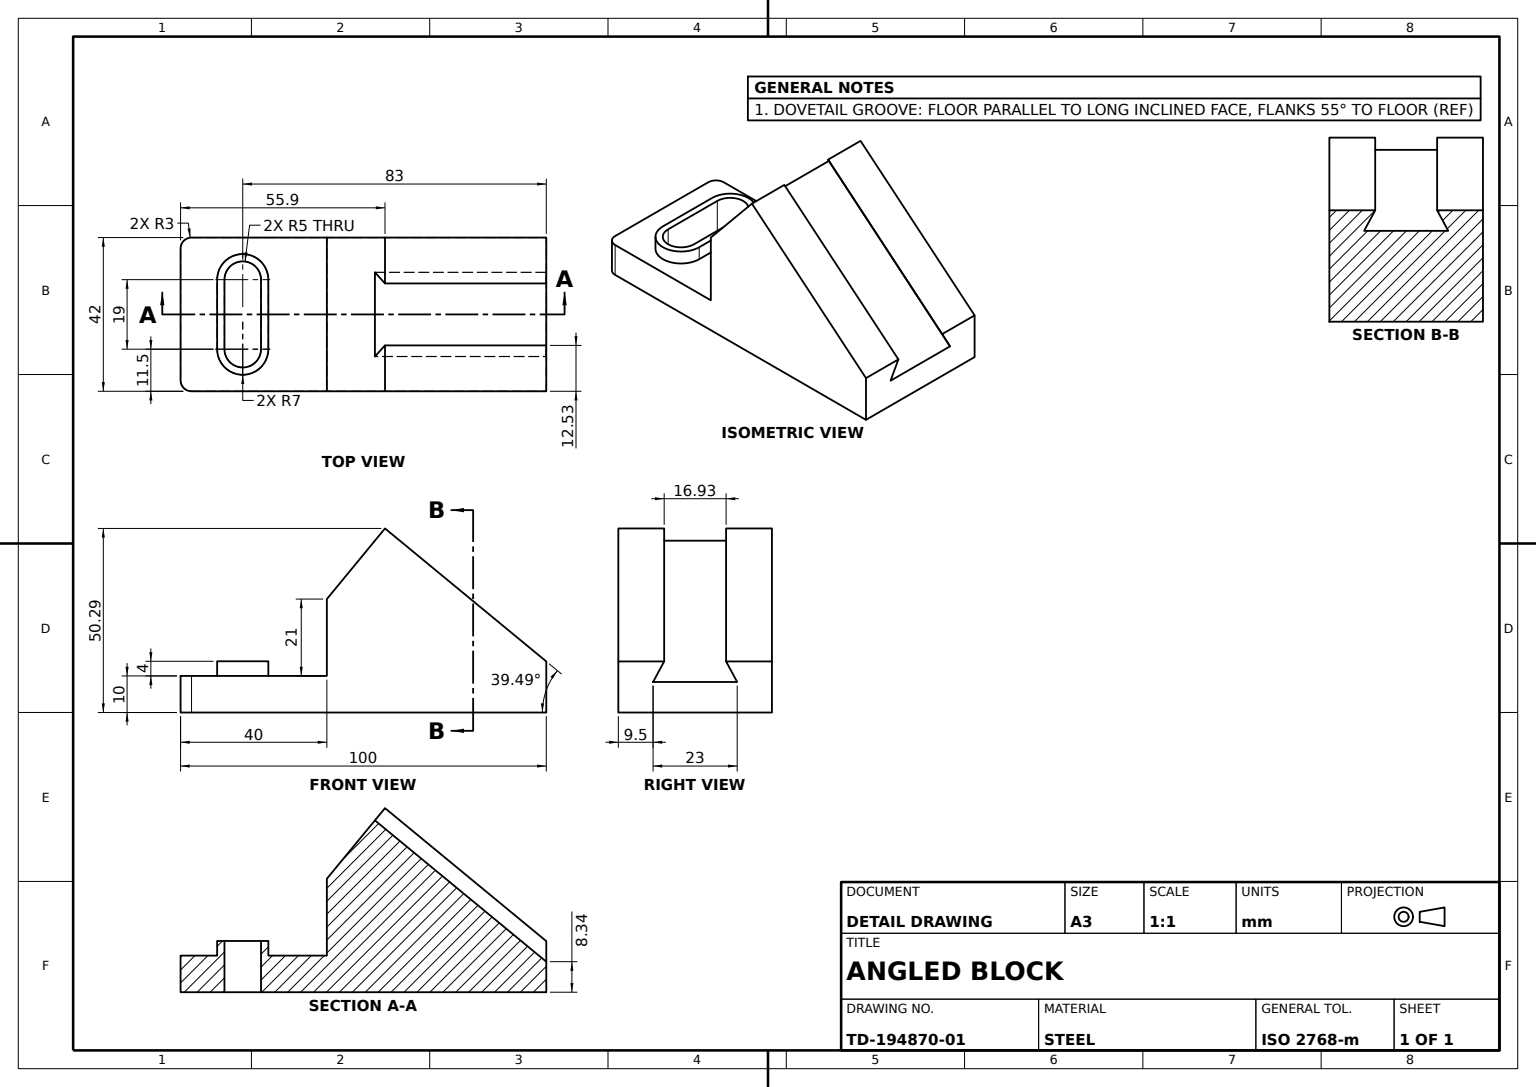
from build123d import *

# Parameters (mm, degrees)
BASE_BLOCK_DEPTH         = 21
SLOT_BOSS_DEPTH          = 4
MOUNTING_START           = -34
MOUNTING_SLOT_DEPTH      = 34
DOVETAIL_GROOVE_55_DEPTH = 464
EDGE_FILLET_R3_R         = 3


with BuildPart() as part:
    # Base Profile Sketch → Base Block (new, symmetric)
    with BuildSketch(Plane.XY):
        Polygon((0, 0), (-100, 0), (-100, 10), (-60, 10), (-60, 31), (-44.102715558, 50.294464164), (0, 22.736028876), align=None)
    extrude(amount=BASE_BLOCK_DEPTH, both=True)

    # Slot Boss Sketch → Slot Boss (add)
    with BuildSketch(Plane(origin=(0, 10, 0), x_dir=(1, 0, 0), z_dir=(0, 1, 0))):
        with BuildLine():
            Line((-90, 9.5), (-90, -9.5))
            ThreePointArc((-90, -9.5), (-83, -16.5), (-76, -9.5))
            Line((-76, -9.5), (-76, 9.5))
            ThreePointArc((-76, 9.5), (-83, 16.5), (-90, 9.5))
        make_face()
        with BuildLine():
            Line((-88, 9.5), (-88, -9.5))
            ThreePointArc((-88, -9.5), (-83, -14.5), (-78, -9.5))
            Line((-78, -9.5), (-78, 9.5))
            ThreePointArc((-78, 9.5), (-83, 14.5), (-88, 9.5))
        make_face(mode=Mode.SUBTRACT)
    extrude(amount=SLOT_BOSS_DEPTH)

    # Mounting Slot Sketch → Mounting Slot (cut)
    with BuildSketch(Plane(origin=(0, 10, 0), x_dir=(1, 0, 0), z_dir=(0, 1, 0)).offset(MOUNTING_START)):
        with BuildLine():
            Line((-88, 9.5), (-88, -9.5))
            ThreePointArc((-88, -9.5), (-83, -14.5), (-78, -9.5))
            Line((-78, -9.5), (-78, 9.5))
            ThreePointArc((-78, 9.5), (-83, 14.5), (-88, 9.5))
        make_face()
    extrude(amount=MOUNTING_SLOT_DEPTH, mode=Mode.SUBTRACT)

    # Dovetail Groove Sketch → Dovetail Groove 55° (cut)
    with BuildSketch(Plane(origin=(-50.952316762, 41.981133327, 0), x_dir=(0, 0, 1), z_dir=(-0.7717785665555229, 0.635891377678218, 0))):
        Polygon((-11.5, 6.439032464), (-8.466266509, 10.771652903), (-21, 10.771652903), (-21, 17.547179775), (21, 17.547179775), (21, 10.771652903), (8.466266509, 10.771652903), (11.5, 6.439032464), align=None)
    extrude(amount=-DOVETAIL_GROOVE_55_DEPTH, mode=Mode.SUBTRACT)

    # Edge Fillet R3
    edge_fillet_r3_edges = [part.edges().sort_by_distance(p)[0] for p in [
        (-100, 5, 21),
        (-100, 5, -21),
    ]]
    fillet(edge_fillet_r3_edges, radius=EDGE_FILLET_R3_R)


solid = part.part
